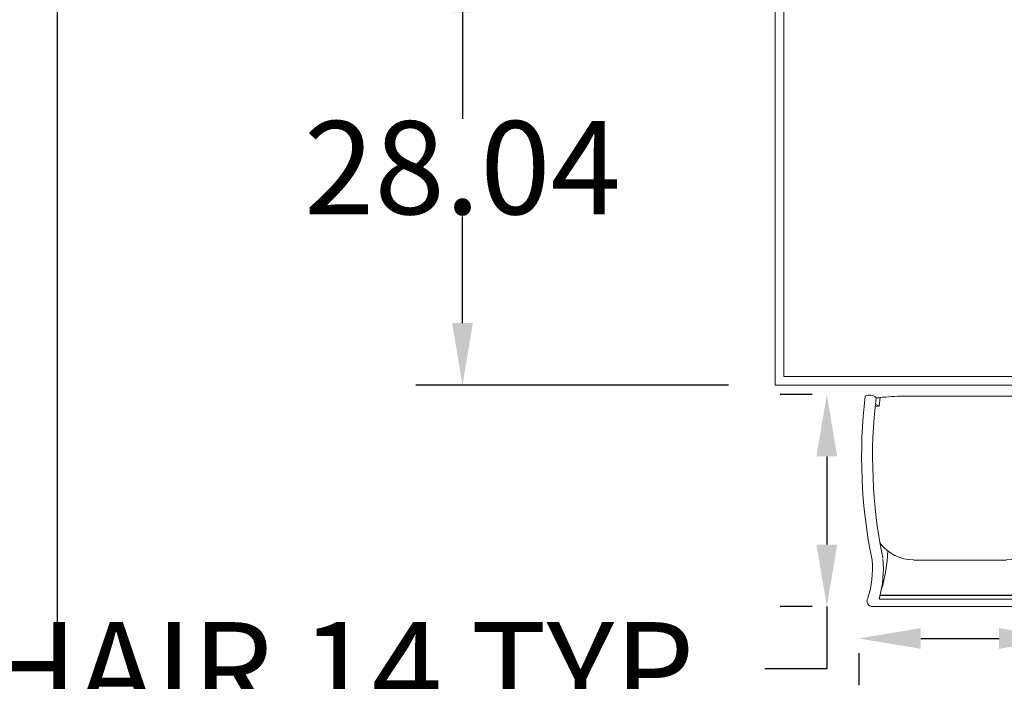
# Model space of a CAD drawing. Units: inches. Extents: x 89 to 490, y -59 to 378.
# Tile 7 of 20: x 275 to 339, y 15 to 58. Entities that reach past the tile are written whole.
import ezdxf

# ---------------------------------------------------------------- set-up
doc = ezdxf.new("R2010")
doc.units = ezdxf.units.IN
doc.header["$MEASUREMENT"] = 0
doc.layers.add('A-ANNO-DIMS', color=2, linetype='Continuous', lineweight=18)
doc.layers.add('Dining Table', color=155, linetype='Continuous', lineweight=18)
doc.styles.get("Standard").update_dxf_attribs({"font": 'arial.ttf'})
doc.dimstyles.get("Standard").update_dxf_attribs({"dimtxt": 6, "dimasz": 4, "dimexe": 3, "dimexo": 3, "dimgap": 0.09, "dimtad": 0, "dimtih": 1, "dimtoh": 1, "dimdec": 1, "dimzin": 0, "dimdsep": 46, "dimlunit": 3, "dimtxsty": 'Standard', "dimcen": 0.09, "dimadec": 0, "dimazin": 0, "dimtfac": 1, "dimtdec": 1, "dimtofl": 0, "dimtmove": 0, "dimatfit": 3, "dimfxl": 1, "dimtolj": 1, "dimtzin": 0, "dimarcsym": 0})

# ---------------------------------------------------------------- blocks, each defined once
blk = doc.blocks.new('A$C51F1')
at = {"color": 0}
for p, q in [((0.2273, 0.4758), (0.0436, 0.4758)), ((0.2273, 0.4758), (0.4111, 0.4758)), ((0.2273, 0.4676), (0.0439, 0.4676)), ((0.2273, 0.4668), (0.0439, 0.4668)), ((0.2273, 0.4676), (0.4107, 0.4676)), ((0.2273, 0.4668), (0.4107, 0.4668)), ((0.2273, 0.3858), (0.1205, 0.3858)), ((0.2273, 0.3858), (0.3341, 0.3858)), ((0.0417, 0.0321), (0.0321, 0.0321)), ((0.0417, 0.0321), (0.0326, 0.0278)), ((0.0435, 0.0127), (0.0417, 0.0321)), ((0.4112, 0.0127), (0.4129, 0.0321)), ((0.4129, 0.0321), (0.4225, 0.0321)), ((0.4129, 0.0321), (0.4221, 0.0278))]:
    blk.add_line(p, q, dxfattribs=at)
blk.add_lwpolyline([(0.4387, 0.4737, 0.102523), (0.4291, 0.3863, -0.080461), (0.4447, 0.0091, -0.3023), (0.4203, 0.012, 0.197932), (0.4111, 0.0127, -0.028193), (0.3571, 0.0091), (0.227, 0.0091), (0.097, 0.0091, -0.028193), (0.0429, 0.0127, 0.197932), (0.0338, 0.012, -0.3023), (0.0093, 0.0091, -0.080461), (0.0249, 0.3863, 0.102523), (0.0153, 0.4737, -0.587111), (0.0261, 0.4929), (0.4279, 0.4929, -0.587111)], format="xyb", close=True, dxfattribs=at)
for centre, radius, start, end in [((0.044, 0.4735), 0.00242, 100.345, 201.3742), ((0.4106, 0.4735), 0.00242, 338.6258, 79.655), ((-0.1898, 0.4063), 0.2409, 354.5513, 15.9626), ((0.0439, 0.4669), 0.000725, 87.3762, 197.5208), ((0.0438, 0.4664), 0.000433, 71.7715, 189.2202), ((-0.2563, 0.3584), 0.3173, 1.1591, 17.5641), ((0.7109, 0.3584), 0.3173, 162.4359, 178.8409), ((0.6445, 0.4063), 0.2409, 164.0374, 185.4487), ((0.4107, 0.4669), 0.000725, 342.4792, 92.6238), ((0.4109, 0.4664), 0.000433, 350.7798, 108.2285), ((0.1214, 0.2879), 0.0978, 90.5164, 143.1927), ((0.3332, 0.2879), 0.0978, 36.8073, 89.4836), ((1.1806, 0.1494), 1.1544, 168.4357, 186.8363), ((-0.7259, 0.1494), 1.1544, 353.1637, 11.5643), ((0.0397, 0.0013), 0.012, 71.7536, 116.5375), ((0.4149, 0.0013), 0.012, 63.4625, 108.2464)]:
    blk.add_arc(centre, radius, start, end, dxfattribs=at)
blk = doc.blocks.new('*D28')
at = {"layer": 'A-ANNO-DIMS', "color": 0, "lineweight": -2, "transparency": 16777216}
for p, q in [((326.431, 33.398), (324.379, 33.398)), ((327.379, 29.398), (327.379, 23.72)), ((326.431, 19.72), (324.379, 19.72)), ((327.379, 19.72), (327.379, 15.72)), ((327.379, 15.72), (323.379, 15.72))]:
    blk.add_line(p, q, dxfattribs=at)
at = {"layer": 'A-ANNO-DIMS', "color": 0, "transparency": 16777216}
for points in [[(326.712, 29.398), (328.046, 29.398), (327.379, 33.398)], [(326.712, 23.72), (328.046, 23.72), (327.379, 19.72)]]:
    blk.add_solid(points, dxfattribs=at)
at = {"layer": 'Defpoints', "color": 0, "transparency": 16777216}
for p in [(329.431, 33.398), (327.379, 19.72), (329.431, 19.72)]:
    blk.add_point(p, dxfattribs=at)
at = {"layer": 'A-ANNO-DIMS', "color": 0, "transparency": 16777216, "insert": (294.517, 15.72), "char_height": 6, "attachment_point": 5}
blk.add_mtext('\\A1;CHAIR 14 TYP.', dxfattribs=at)
blk = doc.blocks.new('*D29')
at = {"layer": 'A-ANNO-DIMS', "color": 0, "lineweight": -2, "transparency": 16777216}
for p, q in [((333.431, 17.668), (338.483, 17.668)), ((342.483, 17.668), (346.483, 17.668)), ((329.431, 16.72), (329.431, 14.668)), ((342.483, 16.72), (342.483, 14.668))]:
    blk.add_line(p, q, dxfattribs=at)
at = {"layer": 'A-ANNO-DIMS', "color": 0, "transparency": 16777216}
for points in [[(333.431, 18.335), (333.431, 17.001), (329.431, 17.668)], [(338.483, 18.335), (338.483, 17.001), (342.483, 17.668)]]:
    blk.add_solid(points, dxfattribs=at)
at = {"layer": 'Defpoints', "color": 0, "transparency": 16777216}
for p in [(329.431, 19.72), (342.483, 19.72), (342.483, 17.668)]:
    blk.add_point(p, dxfattribs=at)
at = {"layer": 'A-ANNO-DIMS', "color": 0, "transparency": 16777216, "insert": (360.893, 17.668), "char_height": 6, "attachment_point": 5}
blk.add_mtext('\\A1;13 TYP.', dxfattribs=at)
blk = doc.blocks.new('*D67')
at = {"layer": 'A-ANNO-DIMS', "color": 0, "lineweight": -2, "transparency": 16777216}
for p, q in [((321.041, 62.023), (300.891, 62.023)), ((303.891, 58.023), (303.891, 51.158)), ((303.891, 37.986), (303.891, 44.851)), ((321.041, 33.986), (300.891, 33.986))]:
    blk.add_line(p, q, dxfattribs=at)
at = {"layer": 'A-ANNO-DIMS', "color": 0, "transparency": 16777216}
for points in [[(303.224, 58.023), (304.558, 58.023), (303.891, 62.023)], [(303.224, 37.986), (304.558, 37.986), (303.891, 33.986)]]:
    blk.add_solid(points, dxfattribs=at)
at = {"layer": 'Defpoints', "color": 0, "transparency": 16777216}
for p in [(303.891, 62.023), (324.041, 62.023), (324.041, 33.986)]:
    blk.add_point(p, dxfattribs=at)
at = {"layer": 'A-ANNO-DIMS', "color": 0, "transparency": 16777216, "insert": (303.891, 48.004), "char_height": 6, "attachment_point": 5}
blk.add_mtext('\\A1;28.04', dxfattribs=at)
blk = doc.blocks.new('*D74')
at = {"layer": 'A-ANNO-DIMS', "color": 0, "lineweight": -2, "transparency": 16777216}
for p, q in [((249.441, 341.741), (249.441, -49.809)), ((277.753, 341.347), (277.753, -49.809)), ((253.441, -46.809), (253.912, -46.809)), ((273.753, -46.809), (273.283, -46.809))]:
    blk.add_line(p, q, dxfattribs=at)
at = {"layer": 'A-ANNO-DIMS', "color": 0, "transparency": 16777216}
for points in [[(253.441, -46.143), (253.441, -47.476), (249.441, -46.809)], [(273.753, -46.143), (273.753, -47.476), (277.753, -46.809)]]:
    blk.add_solid(points, dxfattribs=at)
at = {"layer": 'Defpoints', "color": 0, "transparency": 16777216}
for p in [(249.441, 344.741), (277.753, 344.347), (277.753, -46.809)]:
    blk.add_point(p, dxfattribs=at)
at = {"layer": 'A-ANNO-DIMS', "color": 0, "transparency": 16777216, "insert": (263.597, -46.809), "char_height": 6, "attachment_point": 5}
blk.add_mtext('\\A1;28.31', dxfattribs=at)

msp = doc.modelspace()

# ---------------------------------------------------------------- linework, layer by layer
at = {"layer": 'Dining Table', "ltscale": 0.5}
for points in [[(324.0409, 33.9856), (380.116, 33.9856), (380.116, 62.0232), (324.0409, 62.0232)], [(324.6016, 34.5464), (379.5552, 34.5464), (379.5552, 61.4624), (324.6016, 61.4624)]]:
    msp.add_lwpolyline(points, close=True, dxfattribs=at)

# ---------------------------------------------------------------- block references
at = {"layer": 'Dining Table', "ltscale": 0.5, "xscale": -28.0375393373698, "yscale": 28.0375393373698, "zscale": 28.0375393373698, "rotation": 180}
msp.add_blockref('A$C51F1', (329.592, 33.5401), dxfattribs=at)

# ---------------------------------------------------------------- dimensions: what is measured, and where the dimension line sits
at = {"layer": 'A-ANNO-DIMS'}
dim = msp.add_linear_dim(base=(277.7535, -46.8094), p1=(249.4414, 344.7413), p2=(277.7535, 344.3468), dimstyle='Standard', override={"dimdec": 2, "dimlfac": 1, "dimrnd": 0, "dimzin": 0, "dimdsep": 46, "dimlunit": 2}, dxfattribs=at)
dim.commit()
dim.dimension.update_dxf_attribs({"geometry": '*D74', "text_midpoint": (263.5974, -46.8094)})
dim = msp.add_linear_dim(base=(303.8909, 62.0232), p1=(324.0409, 33.9856), p2=(324.0409, 62.0232), angle=90, dimstyle='Standard', override={"dimdec": 2, "dimlfac": 1, "dimrnd": 0, "dimzin": 0, "dimdsep": 46, "dimlunit": 2}, dxfattribs=at)
dim.commit()
dim.dimension.update_dxf_attribs({"geometry": '*D67', "text_midpoint": (303.8909, 48.0044)})
dim = msp.add_linear_dim(base=(327.3791, 19.7198), p1=(329.4308, 33.3978), p2=(329.4308, 19.7198), angle=270, text='CHAIR <> TYP.', dimstyle='Standard', override={"dimdec": 0, "dimlfac": 1, "dimrnd": 0, "dimzin": 0, "dimdsep": 46, "dimlunit": 2}, dxfattribs=at)
dim.commit()
dim.dimension.update_dxf_attribs({"geometry": '*D28', "text_midpoint": (294.517, 15.7198)})
dim = msp.add_linear_dim(base=(342.4828, 17.668), p1=(329.4308, 19.7198), p2=(342.4828, 19.7198), text='<> TYP.', dimstyle='Standard', override={"dimdec": 0, "dimlfac": 1, "dimrnd": 0, "dimzin": 0, "dimdsep": 46, "dimlunit": 2}, dxfattribs=at)
dim.commit()
dim.dimension.update_dxf_attribs({"geometry": '*D29', "text_midpoint": (360.8934, 17.668)})

doc.saveas('drawing.dxf')
